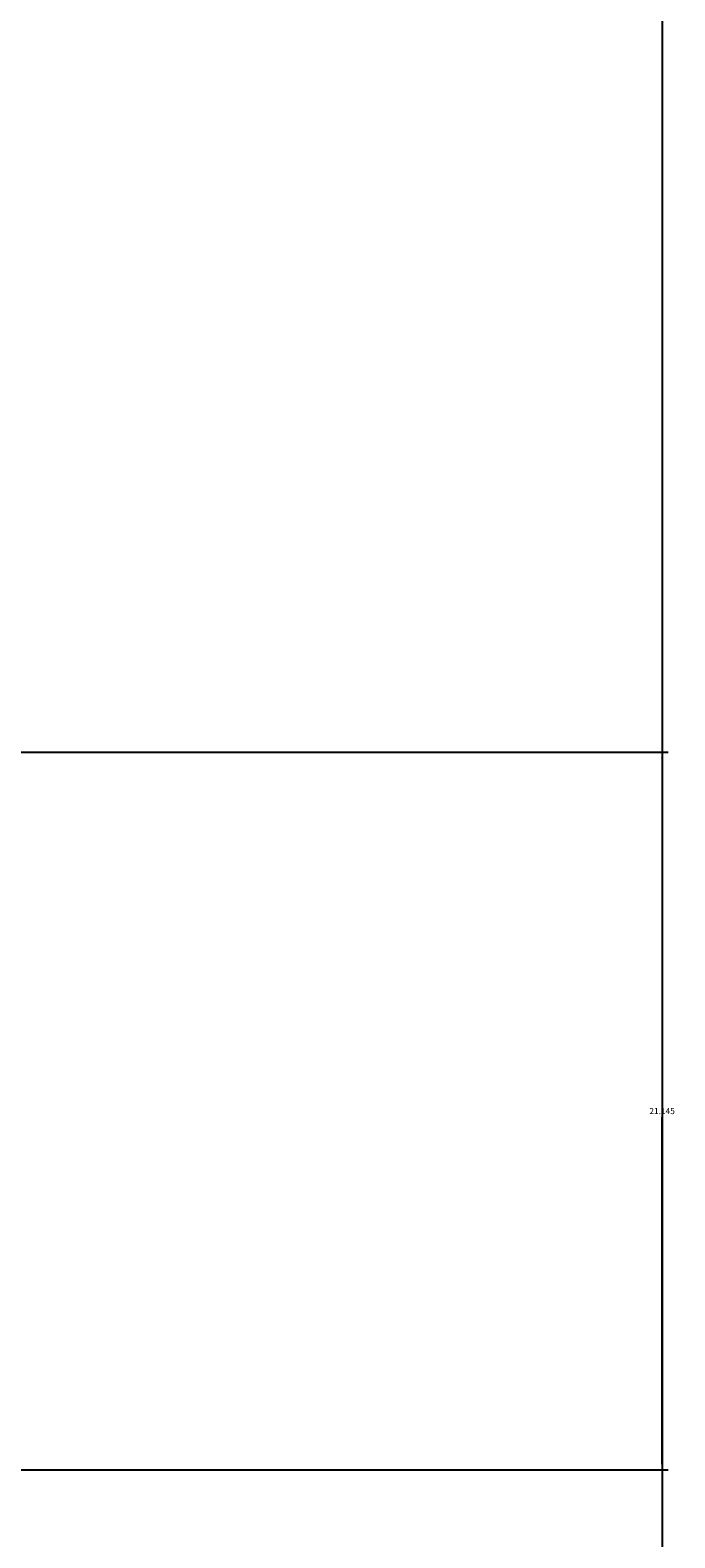
# Model space of a CAD drawing. Units: inches. Extents: x 2307 to 2544, y 2171 to 2540.
# Tile 44 of 52: x 2525 to 2544, y 2438 to 2482. Entities that reach past the tile are written whole.
import ezdxf

# ---------------------------------------------------------------- set-up
doc = ezdxf.new("R2010")
doc.units = ezdxf.units.IN
doc.layers.add('A-ANNO-DIMS', color=2, linetype='Continuous', lineweight=18)
doc.styles.get("Standard").update_dxf_attribs({"font": 'arial.ttf'})
doc.dimstyles.get("Standard").update_dxf_attribs({"dimtxt": 0.18, "dimasz": 0.18, "dimexe": 0.18, "dimexo": 0.0625, "dimgap": 0.09, "dimtad": 0, "dimtih": 1, "dimtoh": 1, "dimdec": 4, "dimzin": 0, "dimdsep": 46, "dimtxsty": 'Standard', "dimcen": 0.09, "dimadec": 0, "dimazin": 0, "dimtfac": 1, "dimtdec": 4, "dimtofl": 0, "dimtmove": 0, "dimatfit": 3, "dimfxl": 1, "dimtolj": 1, "dimtzin": 0, "dimarcsym": 0})

# ---------------------------------------------------------------- blocks, each defined once
blk = doc.blocks.new('*D37')
at = {"layer": 'A-ANNO-DIMS', "color": 0, "lineweight": -2, "transparency": 16777216}
for p, q in [((2524.758, 2520.51), (2544.026, 2520.51)), ((2543.846, 2520.33), (2543.846, 2355.692)), ((2543.846, 2190.69), (2543.846, 2355.328)), ((2524.758, 2190.51), (2544.026, 2190.51))]:
    blk.add_line(p, q, dxfattribs=at)
at = {"layer": 'A-ANNO-DIMS', "color": 0, "transparency": 16777216}
for points in [[(2543.816, 2520.33), (2543.876, 2520.33), (2543.846, 2520.51)], [(2543.816, 2190.69), (2543.876, 2190.69), (2543.846, 2190.51)]]:
    blk.add_solid(points, dxfattribs=at)
at = {"layer": 'Defpoints', "color": 0, "transparency": 16777216}
for p in [(2524.696, 2520.51), (2543.846, 2520.51), (2524.696, 2190.51)]:
    blk.add_point(p, dxfattribs=at)
at = {"layer": 'A-ANNO-DIMS', "color": 0, "transparency": 16777216, "insert": (2543.846, 2355.51), "char_height": 0.18, "attachment_point": 5}
blk.add_mtext('\\A1;330', dxfattribs=at)
blk = doc.blocks.new('*D63')
at = {"layer": 'A-ANNO-DIMS', "color": 0, "lineweight": -2, "transparency": 16777216}
for p, q in [((2505.065, 2460.655), (2544.026, 2460.655)), ((2543.846, 2460.475), (2543.846, 2450.264)), ((2543.846, 2439.69), (2543.846, 2449.9)), ((2515.758, 2439.51), (2544.026, 2439.51))]:
    blk.add_line(p, q, dxfattribs=at)
at = {"layer": 'A-ANNO-DIMS', "color": 0, "transparency": 16777216}
for points in [[(2543.816, 2460.475), (2543.876, 2460.475), (2543.846, 2460.655)], [(2543.816, 2439.69), (2543.876, 2439.69), (2543.846, 2439.51)]]:
    blk.add_solid(points, dxfattribs=at)
at = {"layer": 'Defpoints', "color": 0, "transparency": 16777216}
for p in [(2505.002, 2460.655), (2543.846, 2460.655), (2515.696, 2439.51)]:
    blk.add_point(p, dxfattribs=at)
at = {"layer": 'A-ANNO-DIMS', "color": 0, "transparency": 16777216, "insert": (2543.846, 2450.082), "char_height": 0.18, "attachment_point": 5}
blk.add_mtext('\\A1;21.145', dxfattribs=at)

msp = doc.modelspace()

# ---------------------------------------------------------------- dimensions: what is measured, and where the dimension line sits
at = {"layer": 'A-ANNO-DIMS'}
for base, p1, p2, override, picture, middle in [((2543.8458, 2520.5096), (2524.6958, 2190.5096), (2524.6958, 2520.5096), {"dimdec": 0, "dimlfac": 1, "dimrnd": 0, "dimzin": 0, "dimdsep": 46, "dimlunit": 2}, '*D37', (2543.8458, 2355.5096)), ((2543.8458, 2460.655), (2515.6958, 2439.5096), (2505.002, 2460.655), {"dimdec": 3, "dimlfac": 1, "dimrnd": 0, "dimzin": 0, "dimdsep": 46, "dimlunit": 2}, '*D63', (2543.8458, 2450.0823))]:
    dim = msp.add_linear_dim(base=base, p1=p1, p2=p2, angle=90, dimstyle='Standard', override=override, dxfattribs=at)
    dim.commit()
    dim.dimension.update_dxf_attribs({"geometry": picture, "text_midpoint": middle})

doc.saveas('drawing.dxf')
